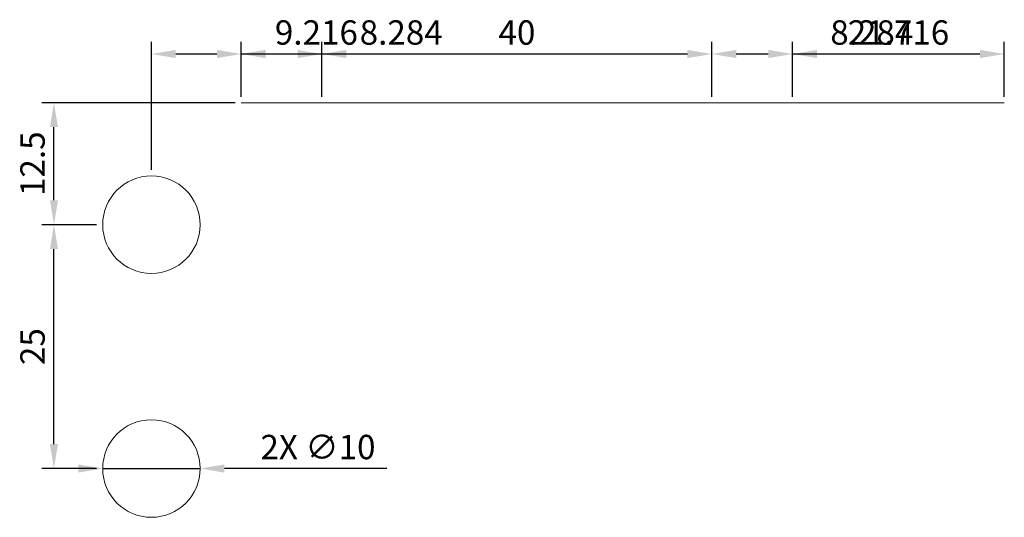
# Model space of a CAD drawing. Units: millimetres. Extents: x -6 to 912, y -42 to 105.
# Tile 2 of 2: x 811 to 912, y -42 to 9. Entities that reach past the tile are written whole.
import ezdxf

# ---------------------------------------------------------------- set-up
doc = ezdxf.new("R2010")
doc.units = ezdxf.units.MM
doc.layers.add('M-CONS', color=8, linetype='Continuous', lineweight=18)
doc.layers.add('M-DIMS', color=2, linetype='Continuous', lineweight=18)
doc.dimstyles.new('ISO-25', dxfattribs={"dimtxt": 2.5, "dimasz": 2.5, "dimexe": 1.25, "dimexo": 0.625, "dimtad": 1, "dimtxsty": 'Standard', "dimcen": 2.5, "dimadec": 0, "dimazin": 0, "dimtfac": 1, "dimtmove": 0, "dimatfit": 3, "dimfxl": 1, "dimarcsym": 0})

# ---------------------------------------------------------------- blocks, each defined once
blk = doc.blocks.new('*D1')
at = {"layer": 'Defpoints', "color": 0, "transparency": 16777216}
for p in [(833.46, 0), (814.24, 0), (819.24, -12.5)]:
    blk.add_point(p, dxfattribs=at)
at = {"layer": 'M-DIMS', "color": 0, "lineweight": -2, "transparency": 16777216}
for p, q in [((832.84, 0), (812.99, 0)), ((814.24, -10), (814.24, -2.5)), ((818.62, -12.5), (812.99, -12.5))]:
    blk.add_line(p, q, dxfattribs=at)
at = {"layer": 'M-DIMS', "color": 0, "transparency": 16777216}
for points in [[(813.83, -2.5), (814.66, -2.5), (814.24, 0)], [(813.83, -10), (814.66, -10), (814.24, -12.5)]]:
    blk.add_solid(points, dxfattribs=at)
at = {"layer": 'M-DIMS', "color": 0, "transparency": 16777216, "insert": (812.37, -6.25), "char_height": 2.5, "attachment_point": 5, "rotation": 90}
blk.add_mtext('12.5', dxfattribs=at)
blk = doc.blocks.new('*D2')
at = {"layer": 'Defpoints', "color": 0, "transparency": 16777216}
for p in [(814.24, -12.5), (819.24, -12.5), (819.24, -37.5)]:
    blk.add_point(p, dxfattribs=at)
at = {"layer": 'M-DIMS', "color": 0, "lineweight": -2, "transparency": 16777216}
for p, q in [((818.62, -12.5), (812.99, -12.5)), ((814.24, -35), (814.24, -15)), ((818.62, -37.5), (812.99, -37.5))]:
    blk.add_line(p, q, dxfattribs=at)
at = {"layer": 'M-DIMS', "color": 0, "transparency": 16777216}
for points in [[(813.83, -15), (814.66, -15), (814.24, -12.5)], [(813.83, -35), (814.66, -35), (814.24, -37.5)]]:
    blk.add_solid(points, dxfattribs=at)
at = {"layer": 'M-DIMS', "color": 0, "transparency": 16777216, "insert": (812.37, -25), "char_height": 2.5, "attachment_point": 5, "rotation": 90}
blk.add_mtext('25', dxfattribs=at)
blk = doc.blocks.new('*D3')
at = {"layer": 'Defpoints', "color": 0, "transparency": 16777216}
for p in [(833.46, 5), (833.46, 0), (824.24, -7.5)]:
    blk.add_point(p, dxfattribs=at)
at = {"layer": 'M-DIMS', "color": 0, "lineweight": -2, "transparency": 16777216}
for p, q in [((824.24, -6.88), (824.24, 6.25)), ((833.46, 0.62), (833.46, 6.25)), ((826.74, 5), (830.96, 5)), ((833.46, 5), (846.38, 5))]:
    blk.add_line(p, q, dxfattribs=at)
at = {"layer": 'M-DIMS', "color": 0, "transparency": 16777216}
for points in [[(826.74, 5.42), (826.74, 4.58), (824.24, 5)], [(830.96, 5.42), (830.96, 4.58), (833.46, 5)]]:
    blk.add_solid(points, dxfattribs=at)
at = {"layer": 'M-DIMS', "color": 0, "transparency": 16777216, "insert": (841.17, 6.88), "char_height": 2.5, "attachment_point": 5}
blk.add_mtext('9.216', dxfattribs=at)
blk = doc.blocks.new('*D4')
at = {"layer": 'Defpoints', "color": 0, "transparency": 16777216}
for p in [(841.74, 5), (833.46, 0), (841.74, 0)]:
    blk.add_point(p, dxfattribs=at)
at = {"layer": 'M-DIMS', "color": 0, "lineweight": -2, "transparency": 16777216}
for p, q in [((833.46, 0.62), (833.46, 6.25)), ((841.74, 0.62), (841.74, 6.25)), ((835.96, 5), (839.24, 5)), ((841.74, 5), (855.49, 5))]:
    blk.add_line(p, q, dxfattribs=at)
at = {"layer": 'M-DIMS', "color": 0, "transparency": 16777216}
for points in [[(835.96, 5.42), (835.96, 4.58), (833.46, 5)], [(839.24, 5.42), (839.24, 4.58), (841.74, 5)]]:
    blk.add_solid(points, dxfattribs=at)
at = {"layer": 'M-DIMS', "color": 0, "transparency": 16777216, "insert": (849.87, 6.88), "char_height": 2.5, "attachment_point": 5}
blk.add_mtext('8.284', dxfattribs=at)
blk = doc.blocks.new('*D5')
at = {"layer": 'Defpoints', "color": 0, "transparency": 16777216}
for p in [(881.74, 5), (841.74, 0), (881.74, 0)]:
    blk.add_point(p, dxfattribs=at)
at = {"layer": 'M-DIMS', "color": 0, "lineweight": -2, "transparency": 16777216}
for p, q in [((841.74, 0.62), (841.74, 6.25)), ((881.74, 0.62), (881.74, 6.25)), ((844.24, 5), (879.24, 5))]:
    blk.add_line(p, q, dxfattribs=at)
at = {"layer": 'M-DIMS', "color": 0, "transparency": 16777216}
for points in [[(844.24, 5.42), (844.24, 4.58), (841.74, 5)], [(879.24, 5.42), (879.24, 4.58), (881.74, 5)]]:
    blk.add_solid(points, dxfattribs=at)
at = {"layer": 'M-DIMS', "color": 0, "transparency": 16777216, "insert": (861.74, 6.88), "char_height": 2.5, "attachment_point": 5}
blk.add_mtext('40', dxfattribs=at)
blk = doc.blocks.new('*D6')
at = {"layer": 'Defpoints', "color": 0, "transparency": 16777216}
for p in [(890.03, 5), (881.74, 0), (890.03, 0)]:
    blk.add_point(p, dxfattribs=at)
at = {"layer": 'M-DIMS', "color": 0, "lineweight": -2, "transparency": 16777216}
for p, q in [((881.74, 0.62), (881.74, 6.25)), ((890.03, 0.62), (890.03, 6.25)), ((884.24, 5), (887.53, 5)), ((890.03, 5), (903.78, 5))]:
    blk.add_line(p, q, dxfattribs=at)
at = {"layer": 'M-DIMS', "color": 0, "transparency": 16777216}
for points in [[(884.24, 5.42), (884.24, 4.58), (881.74, 5)], [(887.53, 5.42), (887.53, 4.58), (890.03, 5)]]:
    blk.add_solid(points, dxfattribs=at)
at = {"layer": 'M-DIMS', "color": 0, "transparency": 16777216, "insert": (898.15, 6.88), "char_height": 2.5, "attachment_point": 5}
blk.add_mtext('8.284', dxfattribs=at)
blk = doc.blocks.new('*D7')
at = {"layer": 'Defpoints', "color": 0, "transparency": 16777216}
for p in [(911.74, 5), (890.03, 0), (911.74, 0)]:
    blk.add_point(p, dxfattribs=at)
at = {"layer": 'M-DIMS', "color": 0, "lineweight": -2, "transparency": 16777216}
for p, q in [((890.03, 0.62), (890.03, 6.25)), ((911.74, 0.62), (911.74, 6.25)), ((892.53, 5), (909.24, 5))]:
    blk.add_line(p, q, dxfattribs=at)
at = {"layer": 'M-DIMS', "color": 0, "transparency": 16777216}
for points in [[(892.53, 5.42), (892.53, 4.58), (890.03, 5)], [(909.24, 5.42), (909.24, 4.58), (911.74, 5)]]:
    blk.add_solid(points, dxfattribs=at)
at = {"layer": 'M-DIMS', "color": 0, "transparency": 16777216, "insert": (900.89, 6.88), "char_height": 2.5, "attachment_point": 5}
blk.add_mtext('21.716', dxfattribs=at)
blk = doc.blocks.new('*D11')
at = {"layer": 'Defpoints', "color": 0, "transparency": 16777216}
for p in [(819.24, -37.5), (829.24, -37.5)]:
    blk.add_point(p, dxfattribs=at)
at = {"layer": 'M-DIMS', "color": 0, "lineweight": -2, "transparency": 16777216}
for p, q in [((816.74, -37.5), (814.24, -37.5)), ((819.24, -37.5), (829.24, -37.5)), ((848.41, -37.5), (831.74, -37.5))]:
    blk.add_line(p, q, dxfattribs=at)
at = {"layer": 'M-DIMS', "color": 0, "transparency": 16777216}
for points in [[(816.74, -37.08), (816.74, -37.92), (819.24, -37.5)], [(831.74, -37.08), (831.74, -37.92), (829.24, -37.5)]]:
    blk.add_solid(points, dxfattribs=at)
at = {"layer": 'M-DIMS', "color": 0, "transparency": 16777216, "insert": (841.33, -35.62), "char_height": 2.5, "attachment_point": 5}
blk.add_mtext('2X ∅10', dxfattribs=at)

msp = doc.modelspace()

# ---------------------------------------------------------------- linework, layer by layer
at = {"layer": 'M-CONS', "extrusion": (0, -1, 0)}
for p, q in [((881.7444, 0, 416.399), (911.7444, 0, 416.399)), ((911.7444, 0, 426.399), (890.0287, 0, 426.399)), ((911.7444, 0, 416.399), (911.7444, 0, 426.399))]:
    msp.add_line(p, q, dxfattribs=at)
at = {"layer": 'M-CONS'}
for centre in [(824.2444, -12.5, 426.399), (824.2444, -37.5, 426.399)]:
    msp.add_circle(centre, 5, dxfattribs=at)
at = {"layer": 'M-CONS', "extrusion": (0, -1, 0)}
for radius, start, end in [(30, 19.471221, 160.528779), (20, 0, 180)]:
    msp.add_arc((861.7444, 416.399), radius, start, end, dxfattribs=at)

# ---------------------------------------------------------------- dimensions: what is measured, and where the dimension line sits
at = {"layer": 'M-DIMS'}
for base, p1, p2, override, picture, middle in [((833.4601, 5), (824.2444, -7.5), (833.4601, 0), {"dimdec": 3, "dimlfac": 1, "dimrnd": 0, "dimzin": 0, "dimdsep": 46, "dimlunit": 2}, '*D3', (841.1685, 6.875)), ((841.7444, 5), (833.4601, 0), (841.7444, 0), {"dimdec": 3, "dimlfac": 1, "dimrnd": 0, "dimzin": 0, "dimdsep": 46, "dimlunit": 2}, '*D4', (849.8694, 6.875)), ((881.7444, 5), (841.7444, 0), (881.7444, 0), {"dimdec": 0, "dimlfac": 1, "dimrnd": 0, "dimzin": 0, "dimdsep": 46, "dimlunit": 2}, '*D5', (861.7444, 6.875)), ((890.0287, 5), (881.7444, 0), (890.0287, 0), {"dimdec": 3, "dimlfac": 1, "dimrnd": 0, "dimzin": 0, "dimdsep": 46, "dimlunit": 2}, '*D6', (898.1537, 6.875)), ((911.7444, 5), (890.0287, 0), (911.7444, 0), {"dimdec": 3, "dimlfac": 1, "dimrnd": 0, "dimzin": 0, "dimdsep": 46, "dimlunit": 2}, '*D7', (900.8865, 6.875))]:
    dim = msp.add_linear_dim(base=base, p1=p1, p2=p2, dimstyle='ISO-25', override=override, dxfattribs=at)
    dim.commit()
    dim.dimension.update_dxf_attribs({"geometry": picture, "text_midpoint": middle})
for base, p1, p2, override, picture, middle in [((814.2444, 0), (819.2444, -12.5), (833.4601, 0), {"dimdec": 1, "dimlfac": 1, "dimrnd": 0, "dimzin": 0, "dimdsep": 46, "dimlunit": 2}, '*D1', (812.3694, -6.25)), ((814.2444, -12.5), (819.2444, -37.5), (819.2444, -12.5), {"dimdec": 0, "dimlfac": 1, "dimrnd": 0, "dimzin": 0, "dimdsep": 46, "dimlunit": 2}, '*D2', (812.3694, -25))]:
    dim = msp.add_linear_dim(base=base, p1=p1, p2=p2, angle=90, dimstyle='ISO-25', override=override, dxfattribs=at)
    dim.commit()
    dim.dimension.update_dxf_attribs({"geometry": picture, "text_midpoint": middle})
dim = msp.add_diameter_dim_2p(p1=(819.2444, -37.5), p2=(829.2444, -37.5), text='2X <>', dimstyle='ISO-25', override={"dimdec": 0, "dimlfac": 1, "dimrnd": 0, "dimzin": 0, "dimdsep": 46, "dimlunit": 2}, dxfattribs=at)
dim.commit()
dim.dimension.update_dxf_attribs({"geometry": '*D11', "text_midpoint": (841.3277, -37.5), "dimtype": 163})

doc.saveas('drawing.dxf')
